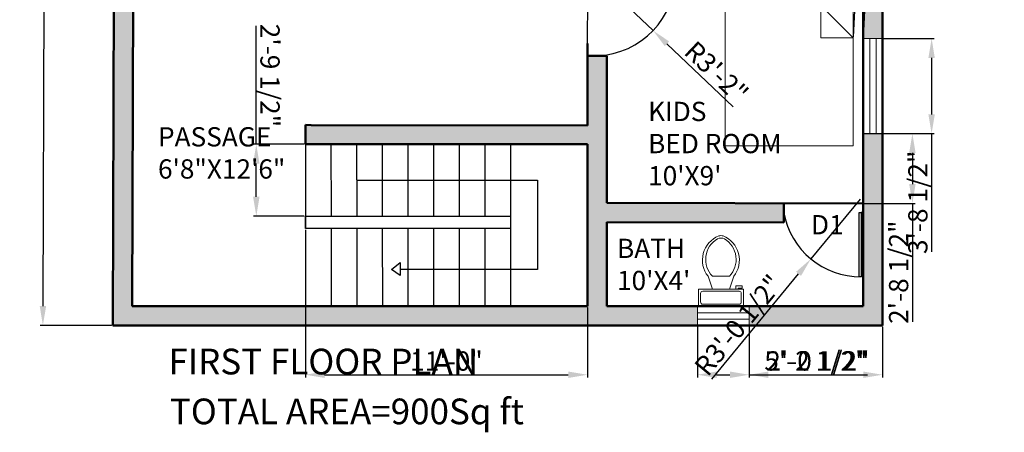
# Model space of a CAD drawing. Units: inches. Extents: x 16989 to 17950, y 7982 to 8536.
# Tile 4 of 5: x 17489 to 17950, y 8049 to 8242. Entities that reach past the tile are written whole.
import ezdxf

# ---------------------------------------------------------------- set-up
doc = ezdxf.new("R2010")
doc.units = ezdxf.units.IN
for name, color, linetype, lineweight in [('A-ANNO-DIMS', 2, 'Continuous', 18), ('A-ANNO-IDEN', 7, 'Continuous', 18), ('A-ANNO-TEXT', 7, 'Continuous', 35), ('A-AREA-IDEN', 7, 'Continuous', 25), ('A-DOOR', 3, 'Continuous', 25), ('A-FLOR-FIXT', 9, 'Continuous', 18), ('A-FLOR-STRS', 7, 'Continuous', 25), ('A-FURN', 8, 'Continuous', 18), ('A-GLAZ', 4, 'Continuous', 18), ('A-WALL', 7, 'Continuous', 50)]:
    doc.layers.add(name, color=color, linetype=linetype, lineweight=lineweight)
doc.layers.add('A-WALL-PATT', color=177, linetype='Continuous', lineweight=13, true_color=0x293189)
doc.styles.get("Standard").update_dxf_attribs({"font": 'arial.ttf'})
doc.dimstyles.new('ISO-25', dxfattribs={"dimtxt": 9, "dimasz": 9, "dimexe": 1.25, "dimexo": 0.625, "dimtad": 1, "dimdec": 1, "dimrnd": 9, "dimlunit": 3, "dimtxsty": 'Standard', "dimcen": 2.5, "dimadec": 0, "dimazin": 0, "dimtfac": 1, "dimtdec": 1, "dimtmove": 0, "dimatfit": 3, "dimfxl": 1, "dimarcsym": 0})

# ---------------------------------------------------------------- blocks, each defined once
blk = doc.blocks.new('*D10')
at = {"layer": 'A-ANNO-DIMS', "color": 0, "lineweight": -2, "transparency": 16777216}
for p, q in [((17533.26, 8460.26), (17499.84, 8460.35)), ((17501.06, 8451.35), (17500.13, 8108.37)), ((17532.27, 8099.28), (17498.85, 8099.37))]:
    blk.add_line(p, q, dxfattribs=at)
at = {"layer": 'A-ANNO-DIMS', "color": 0, "transparency": 16777216}
for points in [[(17499.56, 8451.35), (17502.56, 8451.34), (17501.09, 8460.35)], [(17498.63, 8108.37), (17501.63, 8108.36), (17500.1, 8099.37)]]:
    blk.add_solid(points, dxfattribs=at)
at = {"layer": 'Defpoints', "color": 0, "transparency": 16777216}
for p in [(17533.88, 8460.26), (17500.1, 8099.37), (17532.9, 8099.28)]:
    blk.add_point(p, dxfattribs=at)
at = {"layer": 'A-ANNO-DIMS', "color": 0, "transparency": 16777216, "insert": (17495.37, 8279.87), "char_height": 9, "attachment_point": 5, "rotation": 89.8438}
blk.add_mtext("30'", dxfattribs=at)
blk = doc.blocks.new('Toilet - top')
for p, q in [((9.5, -6), (9.5, -2)), ((-10, -8.5), (-8, -8.5)), ((-10, -9.5), (-10, -8.5)), ((-8, -8.5), (-8, -8)), ((-7, -8), (-7, -9.5)), ((-4, -8), (-6, -14)), ((4, -8), (6, -14)), ((-7, -9.5), (-10, -9.5)), ((4, -14), (-4, -14))]:
    blk.add_line(p, q)
blk.add_lwpolyline([(10.5, -8), (10.5, 0), (-10.5, 0), (-10.5, -8)], close=True)
for points in [[(-9.5, -2), (-9.5, -6)], [(8.5, -1), (-8.5, -1)], [(-8.5, -7), (8.5, -7)]]:
    blk.add_lwpolyline(points)
for centre, radius, start, end in [((-8.62, -1.88), 0.884, 81.8699, 188.1301), ((8.62, -1.88), 0.884, 351.8699, 98.1301), ((-8.62, -6.12), 0.884, 171.8699, 278.1301), ((8.62, -6.12), 0.884, 261.8699, 8.1301), ((3.52, -21.58), 12.17, 141.4691, 247.9714), ((4.2, -21.82), 11.33, 136.3677, 238.9468), ((-3.52, -21.58), 12.17, 292.0284, 38.5307), ((-4.2, -21.82), 11.33, 301.053, 43.6321), ((0, -27.88), 4, 245.7318, 294.2682), ((0, -29), 4, 254.8605, 285.1395)]:
    blk.add_arc(centre, radius, start, end)
blk = doc.blocks.new('Bed - Queen')
for p, q in [((0, -80.00003), (0, 0)), ((0, 0), (59.99999, 0)), ((59.99999, 0), (59.99999, -80.00003)), ((7.99999, -1.2), (28.79998, -1.2)), ((7.99999, -14.4), (7.99999, -1.2)), ((28.79998, -1.2), (28.79998, -14.4)), ((31.19999, -1.2), (51.99999, -1.2)), ((31.19999, -14.4), (31.19999, -1.2)), ((51.99999, -1.2), (51.99999, -16.4)), ((0, -14.4), (44.8, -14.4)), ((44.8, -16.8), (0, -16.8)), ((59.99999, -29.6), (44.8, -14.4)), ((44.8, -14.4), (44.8, -29.6)), ((51.99999, -16.4), (46.79936, -16.4)), ((44.8, -29.6), (59.99999, -29.6)), ((59.99999, -80.00003), (0, -80.00003))]:
    blk.add_line(p, q)
blk = doc.blocks.new('DOOR-LEAF-30IN')
for p, q in [((1, 0), (1, 30)), ((1, 30), (2, 30)), ((2, 30), (2, 0)), ((0, 0), (1, 0)), ((2, 0), (1, 0))]:
    blk.add_line(p, q)
blk = doc.blocks.new('*D57')
at = {"layer": 'A-ANNO-DIMS', "color": 0, "lineweight": -2, "transparency": 16777216}
for p, q in [((17884.52, 8188.92), (17908.1, 8188.92)), ((17906.85, 8179.92), (17906.85, 8165.36)), ((17884.52, 8156.36), (17908.1, 8156.36)), ((17906.85, 8156.36), (17906.85, 8101.06))]:
    blk.add_line(p, q, dxfattribs=at)
at = {"layer": 'A-ANNO-DIMS', "color": 0, "transparency": 16777216}
for points in [[(17905.35, 8179.92), (17908.35, 8179.92), (17906.85, 8188.92)], [(17905.35, 8165.36), (17908.35, 8165.36), (17906.85, 8156.36)]]:
    blk.add_solid(points, dxfattribs=at)
at = {"layer": 'Defpoints', "color": 0, "transparency": 16777216}
for p in [(17883.9, 8188.92), (17883.9, 8156.36), (17906.85, 8156.36)]:
    blk.add_point(p, dxfattribs=at)
at = {"layer": 'A-ANNO-DIMS', "color": 0, "transparency": 16777216, "insert": (17901.57, 8124.21), "char_height": 9, "attachment_point": 5, "rotation": 90}
blk.add_mtext('2\'-8 1/2"', dxfattribs=at)
blk = doc.blocks.new('*D58')
at = {"layer": 'A-ANNO-DIMS', "color": 0, "lineweight": -2, "transparency": 16777216}
for p, q in [((17893.52, 8233.34), (17917.1, 8233.34)), ((17915.85, 8224.34), (17915.85, 8197.92)), ((17893.52, 8188.92), (17917.1, 8188.92)), ((17915.85, 8188.92), (17915.85, 8133.78))]:
    blk.add_line(p, q, dxfattribs=at)
at = {"layer": 'A-ANNO-DIMS', "color": 0, "transparency": 16777216}
for points in [[(17914.35, 8224.34), (17917.35, 8224.34), (17915.85, 8233.34)], [(17914.35, 8197.92), (17917.35, 8197.92), (17915.85, 8188.92)]]:
    blk.add_solid(points, dxfattribs=at)
at = {"layer": 'Defpoints', "color": 0, "transparency": 16777216}
for p in [(17892.9, 8233.34), (17892.9, 8188.92), (17915.85, 8188.92)]:
    blk.add_point(p, dxfattribs=at)
at = {"layer": 'A-ANNO-DIMS', "color": 0, "transparency": 16777216, "insert": (17910.57, 8156.85), "char_height": 9, "attachment_point": 5, "rotation": 90}
blk.add_mtext('3\'-8 1/2"', dxfattribs=at)
blk = doc.blocks.new('*D59')
at = {"layer": 'A-ANNO-DIMS', "color": 0, "lineweight": -2, "transparency": 16777216}
for p, q in [((17806.25, 8098.65), (17806.25, 8075.05)), ((17830.51, 8098.65), (17830.51, 8075.05)), ((17815.25, 8076.3), (17821.51, 8076.3)), ((17830.51, 8076.3), (17885.81, 8076.3))]:
    blk.add_line(p, q, dxfattribs=at)
at = {"layer": 'A-ANNO-DIMS', "color": 0, "transparency": 16777216}
for points in [[(17815.25, 8077.8), (17815.25, 8074.8), (17806.25, 8076.3)], [(17821.51, 8077.8), (17821.51, 8074.8), (17830.51, 8076.3)]]:
    blk.add_solid(points, dxfattribs=at)
at = {"layer": 'Defpoints', "color": 0, "transparency": 16777216}
for p in [(17806.25, 8099.28), (17830.51, 8099.28), (17830.51, 8076.3)]:
    blk.add_point(p, dxfattribs=at)
at = {"layer": 'A-ANNO-DIMS', "color": 0, "transparency": 16777216, "insert": (17862.66, 8081.58), "char_height": 9, "attachment_point": 5}
blk.add_mtext('2\'-0 1/2"', dxfattribs=at)
blk = doc.blocks.new('*D60')
at = {"layer": 'A-ANNO-DIMS', "color": 0, "lineweight": -2, "transparency": 16777216}
for p, q in [((17830.51, 8098.65), (17830.51, 8075.05)), ((17892.9, 8098.65), (17892.9, 8075.05)), ((17839.51, 8076.3), (17883.9, 8076.3))]:
    blk.add_line(p, q, dxfattribs=at)
at = {"layer": 'A-ANNO-DIMS', "color": 0, "transparency": 16777216}
for points in [[(17839.51, 8077.8), (17839.51, 8074.8), (17830.51, 8076.3)], [(17883.9, 8077.8), (17883.9, 8074.8), (17892.9, 8076.3)]]:
    blk.add_solid(points, dxfattribs=at)
at = {"layer": 'Defpoints', "color": 0, "transparency": 16777216}
for p in [(17830.51, 8099.28), (17892.9, 8099.28), (17892.9, 8076.3)]:
    blk.add_point(p, dxfattribs=at)
at = {"layer": 'A-ANNO-DIMS', "color": 0, "transparency": 16777216, "insert": (17861.71, 8081.58), "char_height": 9, "attachment_point": 5}
blk.add_mtext('5\'-2 1/2"', dxfattribs=at)
blk = doc.blocks.new('*D64')
at = {"layer": 'A-ANNO-DIMS', "color": 0, "lineweight": -2, "transparency": 16777216}
for p, q in [((17622.89, 8144.01), (17622.89, 8075.05)), ((17754.9, 8107.65), (17754.9, 8075.05)), ((17631.89, 8076.3), (17745.9, 8076.3))]:
    blk.add_line(p, q, dxfattribs=at)
at = {"layer": 'A-ANNO-DIMS', "color": 0, "transparency": 16777216}
for points in [[(17631.89, 8077.8), (17631.89, 8074.8), (17622.89, 8076.3)], [(17745.9, 8077.8), (17745.9, 8074.8), (17754.9, 8076.3)]]:
    blk.add_solid(points, dxfattribs=at)
at = {"layer": 'Defpoints', "color": 0, "transparency": 16777216}
for p in [(17622.89, 8144.63), (17754.9, 8108.28), (17754.9, 8076.3)]:
    blk.add_point(p, dxfattribs=at)
at = {"layer": 'A-ANNO-DIMS', "color": 0, "transparency": 16777216, "insert": (17688.89, 8081.52), "char_height": 9, "attachment_point": 5}
blk.add_mtext('11\'-0"', dxfattribs=at)
blk = doc.blocks.new('*D65')
at = {"layer": 'A-ANNO-DIMS', "color": 0, "lineweight": -2, "transparency": 16777216}
for p, q in [((17599.93, 8183.96), (17599.92, 8239.26)), ((17622.26, 8183.96), (17598.68, 8183.96)), ((17599.94, 8159.41), (17599.93, 8174.96)), ((17622.26, 8150.41), (17598.69, 8150.41))]:
    blk.add_line(p, q, dxfattribs=at)
at = {"layer": 'A-ANNO-DIMS', "color": 0, "transparency": 16777216}
for points in [[(17601.43, 8174.96), (17598.43, 8174.96), (17599.93, 8183.96)], [(17601.44, 8159.41), (17598.44, 8159.41), (17599.94, 8150.41)]]:
    blk.add_solid(points, dxfattribs=at)
at = {"layer": 'Defpoints', "color": 0, "transparency": 16777216}
for p in [(17599.93, 8183.96), (17622.88, 8183.96), (17622.89, 8150.41)]:
    blk.add_point(p, dxfattribs=at)
at = {"layer": 'A-ANNO-DIMS', "color": 0, "transparency": 16777216, "insert": (17605.2, 8216.11), "char_height": 9, "attachment_point": 5, "rotation": 270.0126}
blk.add_mtext('2\'-9 1/2"', dxfattribs=at)
blk = doc.blocks.new('*D71')
at = {"layer": 'A-ANNO-DIMS', "color": 0, "lineweight": -2, "transparency": 16777216}
for p, q in [((17871.53, 8257.03), (17862.55, 8257.54)), ((17879.26, 8234.23), (17880.59, 8257.77)), ((17880.52, 8256.52), (17885.19, 8256.26)), ((17883.93, 8233.97), (17885.27, 8257.51)), ((17894.18, 8255.75), (17949.24, 8252.63))]:
    blk.add_line(p, q, dxfattribs=at)
at = {"layer": 'A-ANNO-DIMS', "color": 0, "transparency": 16777216}
for points in [[(17871.62, 8258.53), (17871.45, 8255.53), (17880.52, 8256.52)], [(17894.27, 8257.25), (17894.1, 8254.25), (17885.19, 8256.26)]]:
    blk.add_solid(points, dxfattribs=at)
at = {"layer": 'Defpoints', "color": 0, "transparency": 16777216}
for p in [(17885.19, 8256.26), (17879.22, 8233.61), (17883.9, 8233.34)]:
    blk.add_point(p, dxfattribs=at)
at = {"layer": 'A-ANNO-DIMS', "color": 0, "transparency": 16777216, "insert": (17926.5, 8259.21), "char_height": 9, "attachment_point": 5, "rotation": 356.7619}
blk.add_mtext('0\'-4 1/2"', dxfattribs=at)
blk = doc.blocks.new('*D79')
at = {"layer": 'A-ANNO-DIMS', "color": 0, "lineweight": -2, "transparency": 16777216}
for p, q in [((17757.95, 8263.31), (17785.52, 8237.11)), ((17823.06, 8201.44), (17792.04, 8230.91))]:
    blk.add_line(p, q, dxfattribs=at)
at = {"layer": 'A-ANNO-DIMS', "color": 0, "transparency": 16777216}
blk.add_solid([(17793.08, 8232), (17791.01, 8229.83), (17785.52, 8237.11)], dxfattribs=at)
at = {"layer": 'Defpoints', "color": 0, "transparency": 16777216}
for p in [(17757.95, 8263.31), (17785.52, 8237.11)]:
    blk.add_point(p, dxfattribs=at)
at = {"layer": 'A-ANNO-DIMS', "color": 0, "transparency": 16777216, "insert": (17814.41, 8216.86), "char_height": 9, "attachment_point": 5, "rotation": 316.4577}
blk.add_mtext('R3\'-2"', dxfattribs=at)
blk = doc.blocks.new('*D80')
at = {"layer": 'A-ANNO-DIMS', "color": 0, "lineweight": -2, "transparency": 16777216}
for p, q in [((17882.4, 8158.36), (17859.33, 8130.38)), ((17813.04, 8074.25), (17853.6, 8123.44))]:
    blk.add_line(p, q, dxfattribs=at)
at = {"layer": 'A-ANNO-DIMS', "color": 0, "transparency": 16777216}
blk.add_solid([(17852.45, 8124.39), (17854.76, 8122.48), (17859.33, 8130.38)], dxfattribs=at)
at = {"layer": 'Defpoints', "color": 0, "transparency": 16777216}
for p in [(17882.4, 8158.36), (17859.33, 8130.38)]:
    blk.add_point(p, dxfattribs=at)
at = {"layer": 'A-ANNO-DIMS', "color": 0, "transparency": 16777216, "insert": (17826.38, 8098.73), "char_height": 9, "attachment_point": 5, "rotation": 50.488}
blk.add_mtext('R3\'-0 1/2"', dxfattribs=at)

msp = doc.modelspace()

# ---------------------------------------------------------------- hatches: boundary and pattern name
at = {"layer": 'A-WALL-PATT'}
h = msp.add_hatch(color=256, dxfattribs=at)
h.dxf.hatch_style = 1
h.paths.add_polyline_path([(17542.33, 8258.28), (17543.69, 8258.28), (17543.69, 8268.21), (17533.36, 8268.23), (17532.9, 8099.28), (17806.25, 8099.28), (17806.25, 8108.28), (17763.9, 8108.28), (17763.9, 8147.63), (17846.7, 8147.44), (17846.72, 8156.44), (17763.9, 8156.63), (17763.9, 8225.31), (17754.87, 8225.31), (17754.88, 8192.66), (17625.57, 8192.96), (17622.88, 8192.97), (17622.88, 8183.96), (17625.57, 8183.96), (17754.88, 8183.99), (17754.9, 8108.28), (17541.92, 8108.28)])
h.paths.add_polyline_path([(17642.86, 8450.96), (17671.43, 8450.88), (17671.45, 8459.88), (17633.88, 8459.99), (17633.79, 8424.48), (17633.8, 8424.47), (17633.79, 8424.46), (17633.54, 8332.73), (17633.99, 8332.52), (17633.53, 8332.18), (17633.45, 8301.15), (17634.83, 8300.54), (17633.63, 8299.64), (17633.64, 8297.14), (17633.44, 8297.2), (17633.39, 8279.04), (17633.47, 8278.99), (17633.39, 8278.71), (17633.36, 8267.96), (17583.36, 8268.1), (17583.36, 8258.28), (17642.33, 8258.28)])
h.paths.add_polyline_path([(17763.9, 8450.63), (17803.38, 8450.52), (17803.4, 8459.52), (17716.21, 8459.76), (17716.18, 8450.76), (17754.82, 8450.66), (17754.85, 8318.6), (17763.9, 8318.6), (17763.9, 8393.63), (17796.67, 8393.54), (17847.42, 8393.54), (17847.45, 8402.4), (17801.15, 8402.53), (17790.65, 8402.53), (17790.65, 8402.56), (17763.9, 8402.63)])
h.paths.add_polyline_path([(17892.9, 8459.28), (17828.65, 8459.45), (17828.62, 8450.45), (17883.9, 8450.3), (17883.9, 8366.33), (17892.9, 8366.33)])
h.paths.add_polyline_path([(17892.9, 8314.71), (17883.9, 8314.71), (17883.9, 8273.3), (17754.86, 8273.28), (17754.86, 8264.83), (17883.9, 8264.35), (17883.9, 8233.34), (17892.9, 8233.34)])
h.paths.add_polyline_path([(17892.9, 8188.92), (17883.9, 8188.92), (17883.9, 8108.28), (17830.51, 8108.28), (17830.51, 8099.28), (17892.9, 8099.28)])

# ---------------------------------------------------------------- linework, layer by layer
at = {"layer": 'A-DOOR'}
msp.add_line((17754.87, 8231.11), (17755, 8264.83), dxfattribs=at)
for centre, radius, start, end in [((17757.95, 8263.31), 38.03, 272.1614, 0.7533), ((17882.4, 8158.36), 36.26, 190.1857, 270.7901)]:
    msp.add_arc(centre, radius, start, end, dxfattribs=at)
at = {"layer": 'A-FLOR-STRS'}
for p, q in [((17622.88, 8183.96), (17622.89, 8144.63)), ((17634.88, 8183.96), (17634.89, 8150.41)), ((17646.88, 8183.97), (17646.89, 8150.41)), ((17658.88, 8183.97), (17658.89, 8150.41)), ((17670.88, 8183.97), (17670.89, 8150.41)), ((17682.88, 8183.97), (17682.89, 8150.41)), ((17694.88, 8183.98), (17694.89, 8150.41)), ((17706.88, 8183.98), (17706.89, 8150.41)), ((17718.88, 8183.98), (17718.9, 8108.27)), ((17646.89, 8167.19), (17731.52, 8167.19)), ((17731.52, 8167.19), (17731.52, 8125.44)), ((17634.89, 8144.63), (17634.9, 8108.25)), ((17646.89, 8144.63), (17646.9, 8108.26)), ((17658.89, 8144.63), (17658.9, 8108.26)), ((17670.89, 8144.63), (17670.9, 8108.26)), ((17682.89, 8144.63), (17682.9, 8108.26)), ((17694.89, 8144.63), (17694.9, 8108.27)), ((17706.89, 8144.63), (17706.9, 8108.27)), ((17663.18, 8125.44), (17667.31, 8128.79)), ((17667.31, 8122.63), (17663.18, 8125.44)), ((17667.31, 8128.79), (17667.31, 8122.63)), ((17731.52, 8125.44), (17667.31, 8125.44))]:
    msp.add_line(p, q, dxfattribs=at)
msp.add_lwpolyline([(17622.89, 8150.41), (17718.89, 8150.41), (17718.89, 8144.63), (17622.89, 8144.63)], close=True, dxfattribs=at)
at = {"layer": 'A-GLAZ'}
for p, q in [((17892.9, 8233.34), (17883.9, 8233.34)), ((17886.9, 8233.34), (17886.9, 8188.92)), ((17889.9, 8233.34), (17889.9, 8188.92)), ((17892.9, 8188.92), (17883.9, 8188.92)), ((17806.25, 8108.28), (17806.25, 8099.28)), ((17830.51, 8108.28), (17830.51, 8099.28)), ((17830.51, 8105.28), (17806.25, 8105.28)), ((17830.51, 8102.28), (17806.25, 8102.28))]:
    msp.add_line(p, q, dxfattribs=at)
at = {"layer": 'A-WALL'}
for p, q in [((17532.9, 8099.28), (17533.88, 8460.26)), ((17892.9, 8459.28), (17892.9, 8099.28)), ((17883.9, 8264.35), (17883.9, 8108.28)), ((17541.92, 8108.28), (17542.33, 8258.28)), ((17754.87, 8231.11), (17754.88, 8192.66)), ((17763.9, 8225.31), (17754.87, 8225.31)), ((17763.9, 8225.31), (17763.9, 8156.63)), ((17622.88, 8183.96), (17622.88, 8192.97)), ((17622.88, 8192.97), (17625.57, 8192.96)), ((17625.57, 8192.96), (17754.88, 8192.66)), ((17625.57, 8183.96), (17622.88, 8183.96)), ((17625.57, 8183.96), (17754.88, 8183.99)), ((17754.88, 8183.99), (17754.9, 8108.28)), ((17763.9, 8156.63), (17883.9, 8156.36)), ((17846.72, 8156.44), (17846.7, 8147.44)), ((17763.9, 8147.63), (17846.7, 8147.44)), ((17763.9, 8147.63), (17763.9, 8108.28)), ((17532.92, 8108.28), (17532.9, 8108.28)), ((17754.9, 8108.28), (17541.92, 8108.28)), ((17622.9, 8108.28), (17622.9, 8108.25)), ((17883.9, 8108.28), (17763.9, 8108.28)), ((17892.9, 8099.28), (17532.9, 8099.28)), ((17541.9, 8099.25), (17541.9, 8099.28))]:
    msp.add_line(p, q, dxfattribs=at)

# ---------------------------------------------------------------- block references
at = {"layer": 'A-DOOR', "rotation": 180}
msp.add_blockref('DOOR-LEAF-30IN', (17883.9, 8152.1), dxfattribs=at)
at = {"layer": 'A-FLOR-FIXT', "rotation": 180}
msp.add_blockref('Toilet - top', (17817.28, 8108.28), dxfattribs=at)
at = {"layer": 'A-FURN'}
msp.add_blockref('Bed - Queen', (17819.22, 8263.21), dxfattribs=at)

# ---------------------------------------------------------------- texts
at = {"layer": 'A-ANNO-IDEN', "insert": (17859.41, 8150.89), "char_height": 9, "attachment_point": 1}
msp.add_mtext_dynamic_manual_height_columns('D1', width=18.2953, gutter_width=12.5, heights=[0], dxfattribs=at)
at = {"layer": 'A-ANNO-TEXT', "char_height": 12, "attachment_point": 1}
for s, insert in [('FIRST FLOOR PLAN', (17558.88, 8088.46)), ('TOTAL AREA=900Sq ft', (17559.51, 8065.17))]:
    msp.add_mtext_dynamic_manual_height_columns(s, width=318.491, gutter_width=12.5, heights=[0], dxfattribs=dict(at, insert=insert))
at = {"layer": 'A-AREA-IDEN', "char_height": 9, "attachment_point": 1}
for s, insert in [("KIDS\\PBED ROOM\\P10'X9'", (17783.22, 8203.8)), ('PASSAGE\\P6\'8"X12\'6"', (17553.95, 8191.94)), ("BATH\\P10'X4'", (17768.67, 8139.83))]:
    msp.add_mtext_dynamic_manual_height_columns(s, width=78.1764, gutter_width=12.5, heights=[0], dxfattribs=dict(at, insert=insert))

# ---------------------------------------------------------------- dimensions: what is measured, and where the dimension line sits
at = {"layer": 'A-ANNO-DIMS'}
dim = msp.add_aligned_dim(p1=(17533.88, 8460.26), p2=(17532.9, 8099.28), distance=-32.8, dimstyle='ISO-25', override={"dimclrd": 0, "dimclre": 0, "dimclrt": 0}, dxfattribs=at)
dim.commit()
dim.dimension.update_dxf_attribs({"geometry": '*D10', "text_midpoint": (17495.37, 8279.87)})
for base, p1, p2, angle, picture, middle in [((17885.19, 8256.26), (17879.22, 8233.61), (17883.9, 8233.34), 356.7619, '*D71', (17926.5, 8259.21)), ((17599.9318, 8183.9561), (17622.8892, 8150.4124), (17622.8818, 8183.9611), 90.0126, '*D65', (17605.2032, 8216.1068)), ((17915.85, 8188.92), (17892.9, 8233.34), (17892.9, 8188.92), 90, '*D58', (17910.57, 8156.85)), ((17906.85, 8156.36), (17883.9, 8188.92), (17883.9, 8156.36), 270, '*D57', (17901.57, 8124.21))]:
    dim = msp.add_linear_dim(base=base, p1=p1, p2=p2, angle=angle, dimstyle='ISO-25', override={"dimdec": 1, "dimlfac": 1, "dimrnd": 0, "dimzin": 1, "dimdsep": 46, "dimlunit": 4, "dimfrac": 2}, dxfattribs=at)
    dim.commit()
    dim.dimension.update_dxf_attribs({"geometry": picture, "text_midpoint": middle})
for center, mpoint, picture, middle in [((17757.95, 8263.31), (17785.52, 8237.11), '*D79', (17814.41, 8216.86)), ((17882.4, 8158.36), (17859.33, 8130.38), '*D80', (17826.38, 8098.73))]:
    dim = msp.add_radius_dim(center=center, mpoint=mpoint, dimstyle='ISO-25', override={"dimdec": 1, "dimlfac": 1, "dimrnd": 0, "dimzin": 1, "dimdsep": 46, "dimlunit": 4, "dimfrac": 2}, dxfattribs=at)
    dim.commit()
    dim.dimension.update_dxf_attribs({"geometry": picture, "text_midpoint": middle})
for base, p1, p2, picture, middle in [((17754.9, 8076.3), (17622.89, 8144.63), (17754.9, 8108.28), '*D64', (17688.89, 8081.52)), ((17830.51, 8076.3), (17806.25, 8099.28), (17830.51, 8099.28), '*D59', (17862.66, 8081.58)), ((17892.9, 8076.3), (17830.51, 8099.28), (17892.9, 8099.28), '*D60', (17861.71, 8081.58))]:
    dim = msp.add_linear_dim(base=base, p1=p1, p2=p2, dimstyle='ISO-25', override={"dimdec": 1, "dimlfac": 1, "dimrnd": 0, "dimzin": 1, "dimdsep": 46, "dimlunit": 4, "dimfrac": 2}, dxfattribs=at)
    dim.commit()
    dim.dimension.update_dxf_attribs({"geometry": picture, "text_midpoint": middle})

doc.saveas('drawing.dxf')
